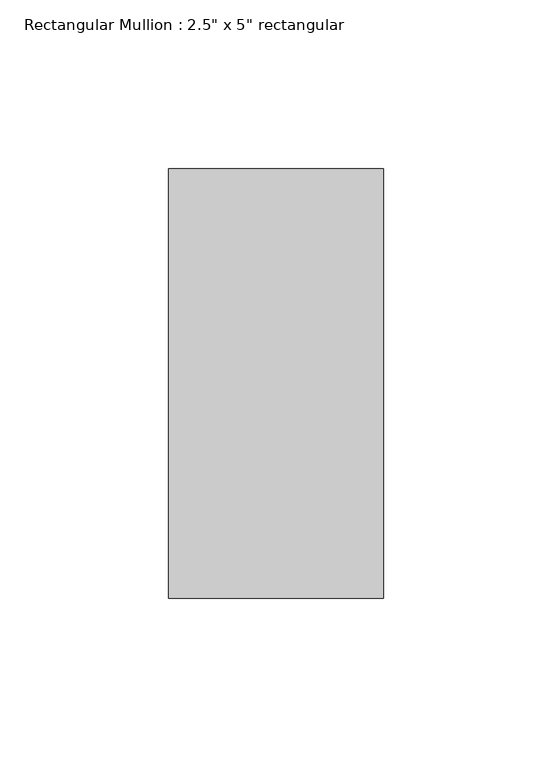
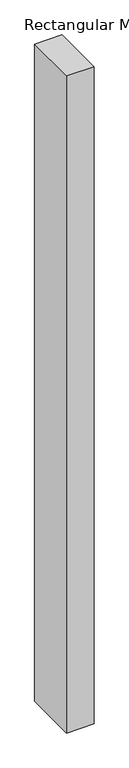
"""IFC4 building model written with IfcOpenShell, lengths in millimetres: member geometry."""

from ifc_helpers import new_model, si_unit, frame, origin, place, context, project, spatial, polyline, outline, extrude, source, transform, mapped, element, save


def member_9c3de6f4(model_context):
    return source(origin(), model_context, "Body", "SweptSolid", [
        extrude(outline(polyline([(31.75, 63.5), (31.75, -63.5), (-31.75, -63.5), (-31.75, 63.5), (31.75, 63.5)])), frame((0.0, 0.0, -1601.4580508), z_axis=(0.0, 0.0, 1.0), x_axis=(1.0, 0.0, 0.0)), (0.0, 0.0, 1.0), 1601.4580508),
    ])


if __name__ == "__main__":
    model = new_model("IFC4")
    model_context = context("Model", 3, world=origin())
    ifc_project = project(units=[si_unit("LENGTHUNIT", "METRE", prefix="MILLI")], contexts=[model_context])
    site = spatial("IfcSite", under=ifc_project)
    building = spatial("IfcBuilding", under=site)
    placement = place(None, origin())
    member_shape = member_9c3de6f4(model_context)
    element("IfcMember", 1, ObjectType="Rectangular Mullion : 2.5\" x 5\" rectangular", at=placement, inside=building, context=model_context, shape_type="MappedRepresentation", body=[
        mapped(member_shape, transform((0.0, 0.0, 0.0), x_axis=(1.0, 0.0, 0.0), y_axis=(0.0, 1.0, 0.0), z_axis=(0.0, 0.0, 1.0))),
    ])
    save(model, "model.ifc")

# Revit data of these elements
# Type "Rectangular Mullion : 2.5\" x 5\" rectangular"
#   built-in parameter 1007304 = 0.416667 (stored number, unit not read)
#   built-in parameter 1007301 = 0.104167 (stored number, unit not read)
#   built-in parameter 1007300 = 0.104167 (stored number, unit not read)
# Element 1 (IfcMember, "Rectangular Mullion : 2.5\" x 5\" rectangular")
#   Materials on its faces: "Aluminum"
# Materials
#   "Aluminum": class "Metal", colour RGB 247 247 247, transparency 0, Description = "Aluminum 6061", Cost = 0
